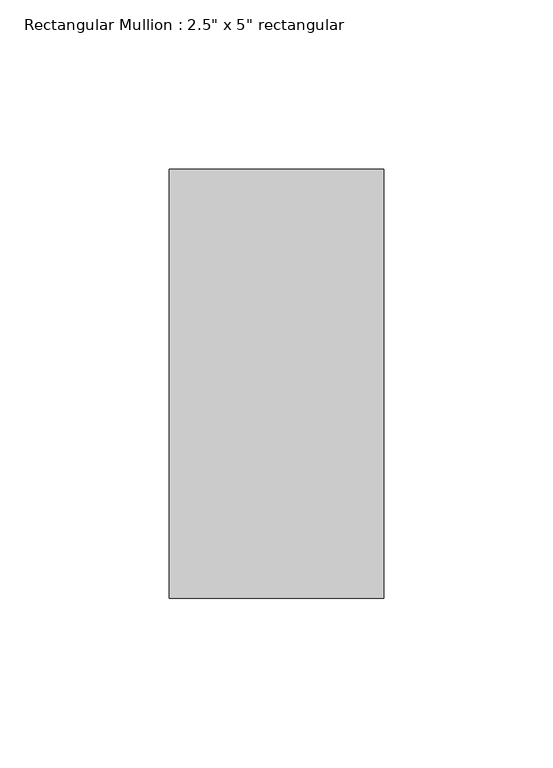
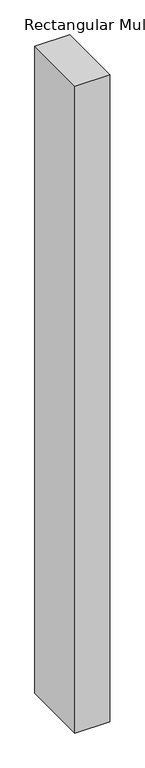
"""IFC4 building model written with IfcOpenShell, lengths in millimetres: member geometry."""

from ifc_helpers import new_model, si_unit, frame, origin, place, context, project, spatial, polyline, outline, extrude, source, transform, mapped, element, save


def member_d635bea1(model_context):
    return source(origin(), model_context, "Body", "SweptSolid", [
        extrude(outline(polyline([(0.0, 63.5), (0.0, -63.5), (-63.5, -63.5), (-63.5, 63.5), (0.0, 63.5)])), frame((0.0, 0.0, -1250.95), z_axis=(0.0, 0.0, 1.0), x_axis=(1.0, 0.0, 0.0)), (0.0, 0.0, 1.0), 1250.95),
    ])


if __name__ == "__main__":
    model = new_model("IFC4")
    model_context = context("Model", 3, world=origin())
    ifc_project = project(units=[si_unit("LENGTHUNIT", "METRE", prefix="MILLI")], contexts=[model_context])
    site = spatial("IfcSite", under=ifc_project)
    building = spatial("IfcBuilding", under=site)
    placement = place(None, origin())
    member_shape = member_d635bea1(model_context)
    element("IfcMember", 1, ObjectType="Rectangular Mullion : 2.5\" x 5\" rectangular", at=placement, inside=building, context=model_context, shape_type="MappedRepresentation", body=[
        mapped(member_shape, transform((0.0, 0.0, 0.0), x_axis=(1.0, 0.0, 0.0), y_axis=(0.0, 1.0, 0.0), z_axis=(0.0, 0.0, 1.0))),
    ])
    save(model, "model.ifc")

# Revit data of these elements
# Type "Rectangular Mullion : 2.5\" x 5\" rectangular"
#   built-in parameter 1007304 = 0.416667 (stored number, unit not read)
#   built-in parameter 1007301 = 0.104167 (stored number, unit not read)
#   built-in parameter 1007300 = 0.104167 (stored number, unit not read)
# Element 1 (IfcMember, "Rectangular Mullion : 2.5\" x 5\" rectangular")
#   Materials on its faces: "Aluminum"
# Materials
#   "Aluminum": class "Metal", colour RGB 247 247 247, transparency 0, Description = "Aluminum 6061", Cost = 0
